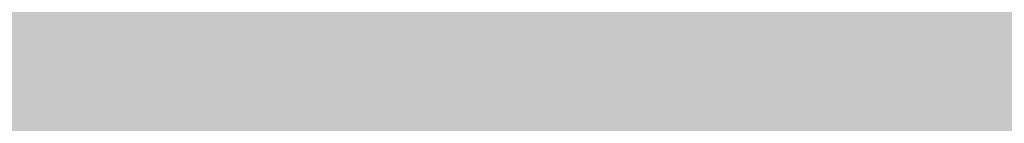
# Model space of a CAD drawing. Units: feet. Extents: x 3168 to 4724, y 827 to 1477.
# Tile 72 of 256: x 3273.2067 to 3273.3412, y 1099.0007 to 1099.0148. Entities that reach past the tile are written whole.
import ezdxf

# ---------------------------------------------------------------- set-up
doc = ezdxf.new("R2010")
doc.units = ezdxf.units.FT
doc.layers.add('A-ELEV', color=7, linetype='Continuous', lineweight=35)
doc.layers.add('A-ELEV-PATT', color=8, linetype='Continuous', lineweight=13)

msp = doc.modelspace()

# ---------------------------------------------------------------- hatches: boundary and pattern name
at = {"layer": 'A-ELEV-PATT'}
h = msp.add_hatch(color=256, dxfattribs=at)
h.dxf.hatch_style = 1
edge = h.paths.add_edge_path()
edge.add_ellipse((3552.90576, 979.22014), major_axis=(36.74492, 0), ratio=0.48484848, start_angle=0, end_angle=360)
edge = h.paths.add_edge_path()
edge.add_ellipse((3559.89164, 929.25228), major_axis=(36.74492, 0), ratio=0.48484848, start_angle=0, end_angle=360)
edge = h.paths.add_edge_path()
edge.add_line((3299.31681, 1198.60608), (3479.91671, 1198.60608))
edge.add_line((3479.91671, 1198.60608), (3479.91671, 1209.86857))
edge.add_spline(control_points=[(3479.91671, 1209.86857), (3464.30116, 1209.86857), (3448.6856, 1209.86857), (3410.94914, 1209.86857), (3388.82823, 1209.86857), (3355.64688, 1209.86857), (3344.58642, 1209.86857), (3327.99574, 1209.86857), (3322.46552, 1209.86857), (3314.17018, 1209.86857), (3311.40507, 1209.86857), (3307.2574, 1209.86857), (3305.87484, 1209.86857), (3303.801, 1209.86857), (3303.10973, 1209.86857), (3302.07281, 1209.86857), (3301.72717, 1209.86857), (3301.20871, 1209.86857), (3301.03589, 1209.86857), (3300.77666, 1209.86857), (3300.69025, 1209.86857), (3300.56064, 1209.86857), (3300.51743, 1209.86857), (3300.45263, 1209.86857), (3300.43102, 1209.86857), (3300.39862, 1209.86857), (3300.38782, 1209.86857), (3300.36622, 1209.86857), (3300.34568, 1209.86857), (3300.34555, 1209.86857), (3300.3455, 1209.86857), (3300.3433, 1209.86857), (3300.34115, 1209.86857), (3300.33791, 1209.86857), (3300.33683, 1209.86857), (3300.33394, 1209.86857), (3300.33213, 1209.86857), (3300.32552, 1209.86858), (3300.32071, 1209.86858), (3300.31092, 1209.86859), (3300.30595, 1209.8686), (3300.29051, 1209.86862), (3300.28005, 1209.86865), (3300.23243, 1209.86878), (3300.1953, 1209.86895), (3299.95107, 1209.87061), (3299.74482, 1209.87433), (3299.43683, 1209.88326), (3299.33439, 1209.88679), (3299.18108, 1209.89292), (3299.13003, 1209.8951), (3298.65222, 1209.9168), (3298.22946, 1209.94572), (3297.60163, 1210.00237), (3297.3934, 1210.02346), (3297.08265, 1210.05831), (3296.97933, 1210.07046), (3296.29295, 1210.15486), (3295.71815, 1210.24336), (3294.86872, 1210.39885), (3294.5877, 1210.45448), (3294.16934, 1210.54335), (3294.03042, 1210.57388), (3291.70715, 1211.1012), (3289.65359, 1211.81344), (3285.77626, 1213.56399), (3283.95141, 1214.60348), (3280.51216, 1216.98008), (3278.89724, 1218.31759), (3276.37991, 1220.82949), (3275.41604, 1221.91774), (3274.03934, 1223.7077), (3273.58104, 1224.34953), (3273.14323, 1225.01632)], knot_values=[39.119033, 39.119033, 39.119033, 39.119033, 39.286353, 39.286353, 39.523379, 39.523379, 39.641892, 39.641892, 39.701148, 39.701148, 39.730777, 39.730777, 39.745591, 39.745591, 39.752998, 39.752998, 39.756701, 39.756701, 39.758553, 39.758553, 39.759479, 39.759479, 39.759942, 39.759942, 39.760173, 39.760173, 39.760289, 39.760289, 39.760405, 39.760405, 39.760463, 39.760463, 39.763389, 39.763389, 39.764851, 39.764851, 39.767304, 39.767304, 39.773825, 39.773825, 39.78057, 39.78057, 39.79477, 39.79477, 39.845194, 39.845194, 40.126715, 40.126715, 40.267476, 40.267476, 40.337856, 40.337856, 40.927023, 40.927023, 41.221606, 41.221606, 41.368898, 41.368898, 42.202622, 42.202622, 42.619485, 42.619485, 42.827916, 42.827916, 46.118323, 46.118323, 49.408731, 49.408731, 52.699139, 52.699139, 54.927489, 54.927489, 56.104228, 56.104228, 56.104228, 56.104228], weights=[1, 1, 1, 1, 1, 1, 1, 1, 1, 1, 1, 1, 1, 1, 1, 1, 1, 1, 1, 1, 1, 1, 1, 1, 1, 1, 1, 1, 1, 1, 1, 1, 1, 1, 1, 1, 1, 1, 1, 1, 1, 1, 1, 1, 1, 1, 1, 1, 1, 1, 1, 1, 1, 1, 1, 1, 1, 1, 1, 1, 1, 1, 1, 1, 1, 1, 1, 1, 1, 1, 1, 1, 1, 1], degree=3, periodic=0)
edge.add_line((3273.14323, 1225.01632), (3273.14323, 1099.01632))
edge.add_line((3273.14323, 1099.01632), (3299.31681, 1099.01632))
edge.add_line((3299.31681, 1099.01632), (3299.31681, 1198.60608))
edge = h.paths.add_edge_path()
edge.add_line((3304.75844, 1324.15806), (3479.91671, 1324.15806))
edge.add_line((3479.91671, 1324.15806), (3479.91671, 1335.71462))
edge.add_line((3479.91671, 1335.71462), (3269.16163, 1335.71462))
edge.add_spline(control_points=[(3269.16163, 1335.71462), (3264.02423, 1335.71462), (3258.36412, 1328.95819), (3259.26431, 1323.90027)], knot_values=[0, 0, 0, 0, 15.412191, 15.412191, 15.412191, 15.412191], degree=3, periodic=0)
edge.add_line((3259.26431, 1323.90027), (3265.51685, 1288.76913))
edge.add_line((3265.51685, 1288.76913), (3275.2651, 1261.54563))
edge.add_line((3275.2651, 1261.54563), (3304.75844, 1261.54563))
edge.add_line((3304.75844, 1261.54563), (3304.75844, 1324.15806))
h = msp.add_hatch(color=256, dxfattribs=at)
h.dxf.hatch_style = 1
h.paths.add_polyline_path([(3384.52525, 1099.01632), (3335.02917, 1099.01632), (3299.31681, 1099.01632), (3273.14323, 1099.01632), (3217.56536, 1099.01632), (3168.06928, 827.11626), (3335.02917, 827.11626)])

# ---------------------------------------------------------------- linework, layer by layer
at = {"layer": 'A-ELEV'}
msp.add_open_spline([(3808.5202, 1099.01632), (3808.5202, 1141.41324), (3808.5202, 1183.81015), (3808.5202, 1226.63532), (3808.5202, 1227.06358), (3808.5202, 1227.49183), (3811.49187, 1248.99467), (3814.46354, 1270.49752), (3817.46523, 1292.21756), (3817.49525, 1292.43476), (3817.52526, 1292.65196), (3817.5728, 1310.10675), (3817.62034, 1327.56153), (3817.66788, 1345.01632), (3817.66788, 1345.45796), (3817.66788, 1345.89961), (3817.66788, 1346.45605), (3817.66788, 1346.57084), (3817.66788, 1346.75289), (3817.66788, 1346.82014), (3817.66788, 1346.93487), (3817.66788, 1346.98234), (3817.66788, 1347.03859), (3817.66788, 1347.04736), (3817.66788, 1347.07366), (3817.66788, 1347.0593), (3817.66788, 1347.06155), (3817.66788, 1347.06267), (3817.66788, 1347.06603), (3817.66787, 1347.06827), (3817.66787, 1347.075), (3817.66787, 1347.07949), (3817.66785, 1347.09294), (3817.66783, 1347.1019), (3817.66777, 1347.12879), (3817.6677, 1347.1467), (3817.66743, 1347.20042), (3817.66716, 1347.23619), (3817.6661, 1347.34338), (3817.66504, 1347.41469), (3817.66081, 1347.62809), (3817.65661, 1347.76971), (3817.63997, 1348.19249), (3817.62351, 1348.47159), (3817.55909, 1349.30007), (3817.49612, 1349.84059), (3817.25543, 1351.42416), (3817.02632, 1352.42879), (3816.30687, 1354.88891), (3815.74375, 1356.26873), (3814.46396, 1358.81921), (3813.74641, 1359.99097), (3812.19584, 1362.17234), (3811.36225, 1363.18212), (3809.58884, 1365.06901), (3808.64882, 1365.94611), (3806.65426, 1367.57962), (3805.5997, 1368.33615), (3803.35289, 1369.72233), (3802.16054, 1370.35239), (3799.60081, 1371.45359), (3798.23269, 1371.92548), (3795.28008, 1372.63462), (3793.69315, 1372.87207), (3791.86944, 1372.92648), (3791.74086, 1372.92922), (3791.35337, 1372.9341), (3791.09271, 1372.9329), (3790.30412, 1372.91507), (3789.76954, 1372.88419), (3789.20919, 1372.83024), (3789.19062, 1372.82842), (3789.13489, 1372.82291), (3789.0977, 1372.81914), (3789.04844, 1372.81401), (3789.0364, 1372.81274), (3789.00026, 1372.80892), (3788.97615, 1372.80633), (3788.9494, 1372.8034), (3788.94679, 1372.80312), (3788.94257, 1372.80266), (3788.94097, 1372.80248), (3788.93857, 1372.80222), (3788.93778, 1372.80213), (3788.93539, 1372.80187), (3788.86753, 1372.7944), (3788.75687, 1372.78223), (3788.70153, 1372.77614), (3788.53553, 1372.75788), (3788.42486, 1372.74571), (3788.09286, 1372.70918), (3787.87152, 1372.68484), (3787.20751, 1372.61179), (3786.76483, 1372.5631), (3785.43681, 1372.41701), (3784.55147, 1372.31962), (3781.89542, 1372.02744), (3780.12473, 1371.83266), (3774.81265, 1371.24831), (3771.27126, 1370.85874), (3760.64709, 1369.69004), (3753.56431, 1368.9109), (3732.31597, 1366.5735), (3718.15042, 1365.01523), (3694.00676, 1362.35933), (3684.02866, 1361.26169), (3674.05056, 1360.16406), (3664.60066, 1360.16406), (3655.15077, 1360.16406), (3626.80108, 1360.16406), (3607.90129, 1360.16406), (3551.20192, 1360.16406), (3513.40234, 1360.16406), (3467.72518, 1360.16406), (3459.8476, 1360.16406), (3436.21487, 1360.16406), (3420.45972, 1360.16406), (3373.19425, 1360.16406), (3341.68395, 1360.16406), (3302.84816, 1360.16406), (3295.52269, 1360.16406), (3286.03829, 1360.16406), (3283.87937, 1360.16406), (3277.40261, 1360.16406), (3273.08477, 1360.16406), (3267.73285, 1360.16406), (3266.69877, 1360.16406), (3263.59652, 1360.16406), (3261.52835, 1360.16406), (3259.23694, 1360.16406), (3259.0137, 1360.16406), (3258.34396, 1360.16406), (3257.89747, 1360.16406), (3257.431, 1360.16406), (3257.41102, 1360.16406), (3257.37057, 1360.16406), (3257.37547, 1360.16406), (3257.3746, 1360.16406), (3257.37394, 1360.16406), (3257.37196, 1360.16406), (3257.37064, 1360.16406), (3257.36667, 1360.16406), (3257.36403, 1360.16406), (3257.35611, 1360.16405), (3257.35083, 1360.16405), (3257.33499, 1360.16402), (3257.32443, 1360.164), (3257.29277, 1360.1639), (3257.27168, 1360.1638), (3257.20844, 1360.1634), (3257.16634, 1360.163), (3257.04021, 1360.16139), (3256.95635, 1360.15978), (3256.7055, 1360.15339), (3256.53924, 1360.14704), (3256.04357, 1360.12192), (3255.7173, 1360.0971), (3254.75245, 1360.00048), (3254.12797, 1359.90651), (3252.18007, 1359.52533), (3250.94157, 1359.14399), (3248.67018, 1358.24329), (3247.63574, 1357.72383), (3245.73263, 1356.60347), (3244.86339, 1356.00206), (3243.25311, 1354.74287), (3242.51197, 1354.08473), (3240.75105, 1352.34478), (3239.80096, 1351.22957), (3238.08777, 1348.87244), (3237.32469, 1347.63036), (3235.98251, 1344.97163), (3235.40221, 1343.55491), (3234.59108, 1340.81546), (3234.31088, 1339.54355), (3233.97649, 1336.80256), (3233.92211, 1335.33088), (3234.14892, 1332.59127), (3234.34953, 1331.3672), (3234.71989, 1329.99937), (3234.75242, 1329.88336), (3234.85362, 1329.5348), (3234.92589, 1329.30168), (3235.02484, 1329.00255), (3235.04692, 1328.93693), (3235.07764, 1328.84724), (3235.08592, 1328.8232), (3235.11094, 1328.75106), (3235.12783, 1328.70296), (3235.14799, 1328.64624), (3235.15106, 1328.63763), (3235.1561, 1328.62353), (3235.15806, 1328.61803), (3235.16021, 1328.61203), (3235.16561, 1328.59694), (3235.1801, 1328.55649), (3235.19026, 1328.5281), (3235.22076, 1328.44295), (3235.24108, 1328.38618), (3235.30207, 1328.21587), (3235.34273, 1328.10232), (3235.4647, 1327.7617), (3235.54601, 1327.53462), (3235.78995, 1326.85338), (3235.95258, 1326.39922), (3236.44046, 1325.03674), (3236.76571, 1324.12841), (3237.74148, 1321.40345), (3238.39198, 1319.5868), (3240.34351, 1314.13687), (3241.64452, 1310.50358), (3245.54757, 1299.60371), (3248.14961, 1292.33713), (3255.95571, 1270.53739), (3261.15977, 1256.00423), (3267.38762, 1238.612), (3268.4114, 1235.75294), (3269.51038, 1232.68386), (3269.58558, 1232.47385), (3269.70661, 1232.13585), (3269.75244, 1232.00786), (3269.82733, 1231.79873), (3269.85638, 1231.7176), (3269.90632, 1231.57812), (3269.92721, 1231.51978), (3269.97247, 1231.39341), (3269.99683, 1231.32537), (3270.0265, 1231.24251), (3270.03181, 1231.22768), (3270.04028, 1231.20402), (3270.03922, 1231.20698), (3270.03936, 1231.2066), (3270.03943, 1231.20641), (3270.03963, 1231.20585), (3270.03977, 1231.20547), (3270.04017, 1231.20433), (3270.04044, 1231.20358), (3270.04125, 1231.20131), (3270.0418, 1231.1998), (3270.04342, 1231.19527), (3270.0445, 1231.19225), (3270.04776, 1231.18318), (3270.04993, 1231.17714), (3270.05644, 1231.15903), (3270.06079, 1231.14696), (3270.07387, 1231.11076), (3270.08261, 1231.08666), (3270.10894, 1231.01441), (3270.1266, 1230.96635), (3270.17993, 1230.82246), (3270.21595, 1230.72692), (3270.32532, 1230.44151), (3270.40003, 1230.25281), (3270.62925, 1229.69144), (3270.78888, 1229.3235), (3271.28649, 1228.23832), (3271.6431, 1227.53975), (3272.77586, 1225.51528), (3273.61417, 1224.2605), (3275.41604, 1221.91774), (3276.37991, 1220.82949), (3278.89724, 1218.31759), (3280.51216, 1216.98008), (3283.95141, 1214.60348), (3285.77626, 1213.56399), (3289.65359, 1211.81344), (3291.70715, 1211.1012), (3294.03042, 1210.57388), (3294.16934, 1210.54335), (3294.5877, 1210.45448), (3294.86872, 1210.39885), (3295.71815, 1210.24336), (3296.29295, 1210.15486), (3296.97933, 1210.07046), (3297.08265, 1210.05831), (3297.3934, 1210.02346), (3297.60163, 1210.00237), (3298.22946, 1209.94572), (3298.65222, 1209.9168), (3299.13003, 1209.8951), (3299.18108, 1209.89292), (3299.33439, 1209.88679), (3299.43683, 1209.88326), (3299.74482, 1209.87433), (3299.95107, 1209.87061), (3300.1953, 1209.86895), (3300.23243, 1209.86878), (3300.28005, 1209.86865), (3300.29051, 1209.86862), (3300.30595, 1209.8686), (3300.31092, 1209.86859), (3300.32071, 1209.86858), (3300.32552, 1209.86858), (3300.33213, 1209.86857), (3300.33394, 1209.86857), (3300.33683, 1209.86857), (3300.33791, 1209.86857), (3300.34115, 1209.86857), (3300.3433, 1209.86857), (3300.3455, 1209.86857), (3300.34555, 1209.86857), (3300.34568, 1209.86857), (3300.36622, 1209.86857), (3300.38782, 1209.86857), (3300.39862, 1209.86857), (3300.43102, 1209.86857), (3300.45263, 1209.86857), (3300.51743, 1209.86857), (3300.56064, 1209.86857), (3300.69025, 1209.86857), (3300.77666, 1209.86857), (3301.03589, 1209.86857), (3301.20871, 1209.86857), (3301.72717, 1209.86857), (3302.07281, 1209.86857), (3303.10973, 1209.86857), (3303.801, 1209.86857), (3305.87484, 1209.86857), (3307.2574, 1209.86857), (3311.40507, 1209.86857), (3314.17018, 1209.86857), (3322.46552, 1209.86857), (3327.99574, 1209.86857), (3344.58642, 1209.86857), (3355.64688, 1209.86857), (3388.82823, 1209.86857), (3410.94914, 1209.86857), (3477.31185, 1209.86857), (3521.55366, 1209.86857), (3566.83618, 1209.86857), (3567.87689, 1209.86857), (3570.99902, 1209.86857), (3573.08043, 1209.86857), (3575.7814, 1209.86857), (3576.40094, 1209.86857), (3577.29582, 1209.86857), (3577.57115, 1209.86857), (3578.39715, 1209.86857), (3578.94781, 1209.86857), (3579.75649, 1209.86857), (3580.01451, 1209.86857), (3580.34274, 1209.86857), (3580.32686, 1209.86857), (3580.32717, 1209.86857), (3580.32732, 1209.86857), (3580.32778, 1209.86857), (3580.32809, 1209.86857), (3580.329, 1209.86857), (3580.32961, 1209.86857), (3580.33145, 1209.86857), (3580.33267, 1209.86857), (3580.33633, 1209.86857), (3580.33878, 1209.86857), (3580.34611, 1209.86856), (3580.35099, 1209.86856), (3580.36566, 1209.86854), (3580.37544, 1209.86852), (3580.4048, 1209.86845), (3580.42439, 1209.86838), (3580.48318, 1209.86808), (3580.52244, 1209.86779), (3580.64036, 1209.86662), (3580.71919, 1209.86545), (3580.95632, 1209.86077), (3581.11522, 1209.85607), (3581.59416, 1209.83723), (3581.91642, 1209.81833), (3582.88995, 1209.74243), (3583.54799, 1209.66617), (3585.53183, 1209.36062), (3586.86722, 1209.05389), (3589.47155, 1208.25247), (3590.74024, 1207.75785), (3591.99545, 1207.1588), (3592.05781, 1207.12874), (3592.24424, 1207.03795), (3592.36768, 1206.97663), (3592.73528, 1206.79036), (3592.97675, 1206.6631), (3593.24454, 1206.51644), (3593.27473, 1206.49982), (3593.36512, 1206.44984), (3593.42511, 1206.41633), (3593.60431, 1206.31529), (3593.72273, 1206.24721), (3593.85721, 1206.1684), (3593.87436, 1206.15832), (3593.92574, 1206.12804), (3593.9599, 1206.1078), (3594.06209, 1206.0469), (3594.12983, 1206.00607), (3594.20844, 1205.95817), (3594.21968, 1205.9513), (3594.25339, 1205.93069), (3594.27582, 1205.91692), (3594.34297, 1205.87554), (3594.38756, 1205.84785), (3594.43362, 1205.81905), (3594.43526, 1205.81802), (3594.44017, 1205.81495), (3594.44345, 1205.81289), (3594.44712, 1205.81059), (3594.44752, 1205.81035), (3594.44869, 1205.80961), (3594.44948, 1205.80912), (3594.45037, 1205.80856), (3594.45047, 1205.8085), (3594.4506, 1205.80842), (3594.4674, 1205.79789), (3594.49327, 1205.78167), (3594.5062, 1205.77357), (3594.54501, 1205.74925), (3594.57088, 1205.73303), (3594.64849, 1205.6844), (3594.70023, 1205.65197), (3594.85544, 1205.55469), (3594.95892, 1205.48984), (3595.26936, 1205.29528), (3595.47631, 1205.16558), (3596.09719, 1204.77646), (3596.5111, 1204.51705), (3597.75284, 1203.73883), (3598.58067, 1203.22001), (3601.06415, 1201.66355), (3602.71981, 1200.62591), (3607.68677, 1197.513), (3610.99809, 1195.43773), (3620.93202, 1189.2119), (3627.55464, 1185.06135), (3647.42251, 1172.60971), (3660.66775, 1164.30861), (3700.40348, 1139.40531), (3726.89397, 1122.80312), (3757.20572, 1103.80605), (3761.02697, 1101.41118), (3764.84822, 1099.01632), (3745.32827, 1099.01632), (3725.80832, 1099.01632), (3706.28837, 1099.01632), (3706.28837, 1108.45324), (3706.28837, 1117.89016), (3706.28837, 1127.32708), (3710.75075, 1127.32708), (3715.21314, 1127.32708), (3719.67553, 1127.32708)], degree=3, knots=[0, 0, 0, 0, 0.982037, 0.982037, 0.991957, 0.991957, 0.991957, 1.966522, 1.966522, 1.976367, 1.976367, 1.976367, 2.976367, 2.976367, 2.976367, 3.00169, 3.00169, 3.008272, 3.008272, 3.012129, 3.012129, 3.014851, 3.014851, 3.015353, 3.015353, 3.016359, 3.016359, 3.017365, 3.017365, 3.019376, 3.019376, 3.023398, 3.023398, 3.031442, 3.031442, 3.047531, 3.047531, 3.079708, 3.079708, 3.144063, 3.144063, 3.272772, 3.272772, 3.53019, 3.53019, 4.045026, 4.045026, 5.074698, 5.074698, 6.700878, 6.700878, 8.327058, 8.327058, 9.953238, 9.953238, 11.579418, 11.579418, 13.205598, 13.205598, 14.831778, 14.831778, 16.457958, 16.457958, 18.084138, 18.084138, 18.206872, 18.206872, 18.45234, 18.45234, 18.943275, 18.943275, 18.960093, 18.960093, 18.993729, 18.993729, 19.00461, 19.00461, 19.026374, 19.026374, 19.028737, 19.028737, 19.03018, 19.03018, 19.030897, 19.030897, 19.032332, 19.032332, 19.033766, 19.033766, 19.036636, 19.036636, 19.042374, 19.042374, 19.053851, 19.053851, 19.076805, 19.076805, 19.122714, 19.122714, 19.21453, 19.21453, 19.398163, 19.398163, 19.765429, 19.765429, 20.024128, 20.024128, 20.024128, 20.092031, 20.092031, 20.227836, 20.227836, 20.499446, 20.499446, 20.556051, 20.556051, 20.66926, 20.66926, 20.895678, 20.895678, 20.948316, 20.948316, 20.963829, 20.963829, 20.994855, 20.994855, 21.002285, 21.002285, 21.017146, 21.017146, 21.01875, 21.01875, 21.021959, 21.021959, 21.022102, 21.022102, 21.022249, 21.022249, 21.022708, 21.022708, 21.023627, 21.023627, 21.025464, 21.025464, 21.029138, 21.029138, 21.036486, 21.036486, 21.051183, 21.051183, 21.080575, 21.080575, 21.139361, 21.139361, 21.256932, 21.256932, 21.492073, 21.492073, 21.962356, 21.962356, 23.01002, 23.01002, 24.057684, 24.057684, 25.105348, 25.105348, 26.153011, 26.153011, 27.776787, 27.776787, 29.400562, 29.400562, 31.024337, 31.024337, 32.278801, 32.278801, 33.533265, 33.533265, 34.467568, 34.467568, 34.553971, 34.553971, 34.726776, 34.726776, 34.775309, 34.775309, 34.793079, 34.793079, 34.82862, 34.82862, 34.834979, 34.834979, 34.839039, 34.839039, 34.839411, 34.839411, 34.840285, 34.840285, 34.842034, 34.842034, 34.845531, 34.845531, 34.852525, 34.852525, 34.866512, 34.866512, 34.894488, 34.894488, 34.950439, 34.950439, 35.062342, 35.062342, 35.286147, 35.286147, 35.733758, 35.733758, 35.821815, 35.821815, 35.828283, 35.828283, 35.832225, 35.832225, 35.834724, 35.834724, 35.836521, 35.836521, 35.838617, 35.838617, 35.839073, 35.839073, 35.839345, 35.839345, 35.839617, 35.839617, 35.840161, 35.840161, 35.841249, 35.841249, 35.843425, 35.843425, 35.847778, 35.847778, 35.856482, 35.856482, 35.873891, 35.873891, 35.908709, 35.908709, 35.978345, 35.978345, 36.117617, 36.117617, 36.396161, 36.396161, 36.953248, 36.953248, 38.067423, 38.067423, 40.295772, 40.295772, 42.524122, 42.524122, 45.81453, 45.81453, 49.104937, 49.104937, 52.395345, 52.395345, 52.603776, 52.603776, 53.020639, 53.020639, 53.854363, 53.854363, 54.001655, 54.001655, 54.296238, 54.296238, 54.885405, 54.885405, 54.955785, 54.955785, 55.096546, 55.096546, 55.378067, 55.378067, 55.42849, 55.42849, 55.442691, 55.442691, 55.449436, 55.449436, 55.455957, 55.455957, 55.458409, 55.458409, 55.459872, 55.459872, 55.462798, 55.462798, 55.462856, 55.462856, 55.462972, 55.462972, 55.463088, 55.463088, 55.463319, 55.463319, 55.463782, 55.463782, 55.464708, 55.464708, 55.46656, 55.46656, 55.470263, 55.470263, 55.47767, 55.47767, 55.492484, 55.492484, 55.522112, 55.522112, 55.581369, 55.581369, 55.699882, 55.699882, 55.936907, 55.936907, 56.410959, 56.410959, 56.42211, 56.42211, 56.444413, 56.444413, 56.451051, 56.451051, 56.454001, 56.454001, 56.459901, 56.459901, 56.462666, 56.462666, 56.463418, 56.463418, 56.464171, 56.464171, 56.465675, 56.465675, 56.468684, 56.468684, 56.474702, 56.474702, 56.486738, 56.486738, 56.51081, 56.51081, 56.558955, 56.558955, 56.655243, 56.655243, 56.847821, 56.847821, 57.232975, 57.232975, 58.003284, 58.003284, 59.543901, 59.543901, 62.625137, 62.625137, 68.787607, 68.787607, 74.950078, 74.950078, 75.27336, 75.27336, 75.919923, 75.919923, 77.213051, 77.213051, 77.377769, 77.377769, 77.707206, 77.707206, 78.366079, 78.366079, 78.462532, 78.462532, 78.655436, 78.655436, 79.041245, 79.041245, 79.105735, 79.105735, 79.234714, 79.234714, 79.492672, 79.492672, 79.502197, 79.502197, 79.521249, 79.521249, 79.523534, 79.523534, 79.528103, 79.528103, 79.528682, 79.528682, 79.528885, 79.528885, 79.529089, 79.529089, 79.529495, 79.529495, 79.530308, 79.530308, 79.531935, 79.531935, 79.535187, 79.535187, 79.541693, 79.541693, 79.554704, 79.554704, 79.580725, 79.580725, 79.632769, 79.632769, 79.736856, 79.736856, 79.94503, 79.94503, 80.361377, 80.361377, 80.421435, 80.421435, 80.421435, 81.421435, 81.421435, 81.421435, 82.421435, 82.421435, 82.421435, 83.421435, 83.421435, 83.421435, 83.421435], dxfattribs=at)

doc.saveas('drawing.dxf')
